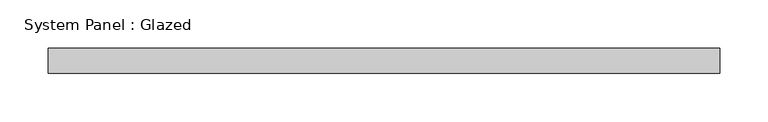
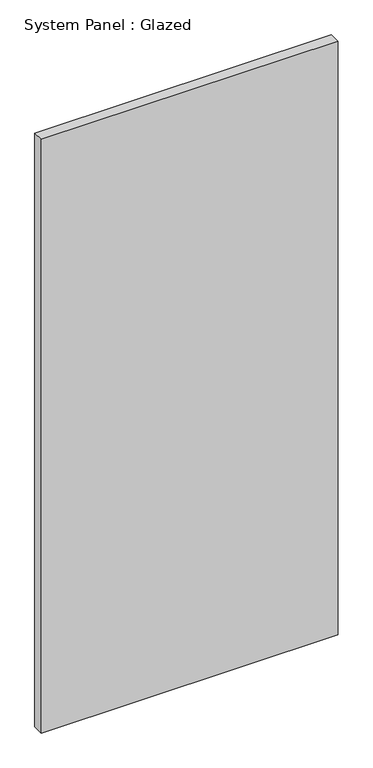
"""IFC4 building model written with IfcOpenShell, lengths in millimetres: plate geometry, System Panel : Glazed."""

from ifc_helpers import new_model, si_unit, origin, origin_with_axes, place, context, project, spatial, polyline, outline, extrude, source, transform, mapped, element, save


def system_panel_glazed_d989bf7f(model_context):
    return source(origin(), model_context, "Body", "SweptSolid", [
        extrude(outline(polyline([(346.075, 19.05), (-346.075, 19.05), (-346.075, 44.45), (346.075, 44.45), (346.075, 19.05)])), origin_with_axes(), (0.0, 0.0, 1.0), 1462.6963029),
    ])


if __name__ == "__main__":
    model = new_model("IFC4")
    model_context = context("Model", 3, world=origin())
    ifc_project = project(units=[si_unit("LENGTHUNIT", "METRE", prefix="MILLI")], contexts=[model_context])
    site = spatial("IfcSite", under=ifc_project)
    building = spatial("IfcBuilding", under=site)
    placement = place(None, origin())
    system_panel_glazed_shape = system_panel_glazed_d989bf7f(model_context)
    element("IfcPlate", 1, ObjectType="System Panel : Glazed", at=placement, inside=building, context=model_context, shape_type="MappedRepresentation", body=[
        mapped(system_panel_glazed_shape, transform((0.0, 0.0, 0.0), x_axis=(1.0, 0.0, 0.0), y_axis=(0.0, 1.0, 0.0), z_axis=(0.0, 0.0, 1.0))),
    ])
    save(model, "model.ifc")

# Revit data of these elements
# Type "System Panel : Glazed"
#   Construction Type Id = "GSP4R"
#   Analytic Construction = "1/8 in Pilkington single glazing"
#   Visual Light Transmittance = 0.9
#   Solar Heat Gain Coefficient = 0.86
#   Heat Transfer Coefficient (U) = 1.18115 BTU/(h·ft²·°F)
#   Define Thermal Properties by = 1
# Element 1 (IfcPlate, "System Panel : Glazed")
#   Materials on its faces: "Glass"
# Materials
#   "Glass": class "Glass", colour RGB 0 128 192, transparency 0.75, Description = "Soda Lime Glass", Cost = 0
